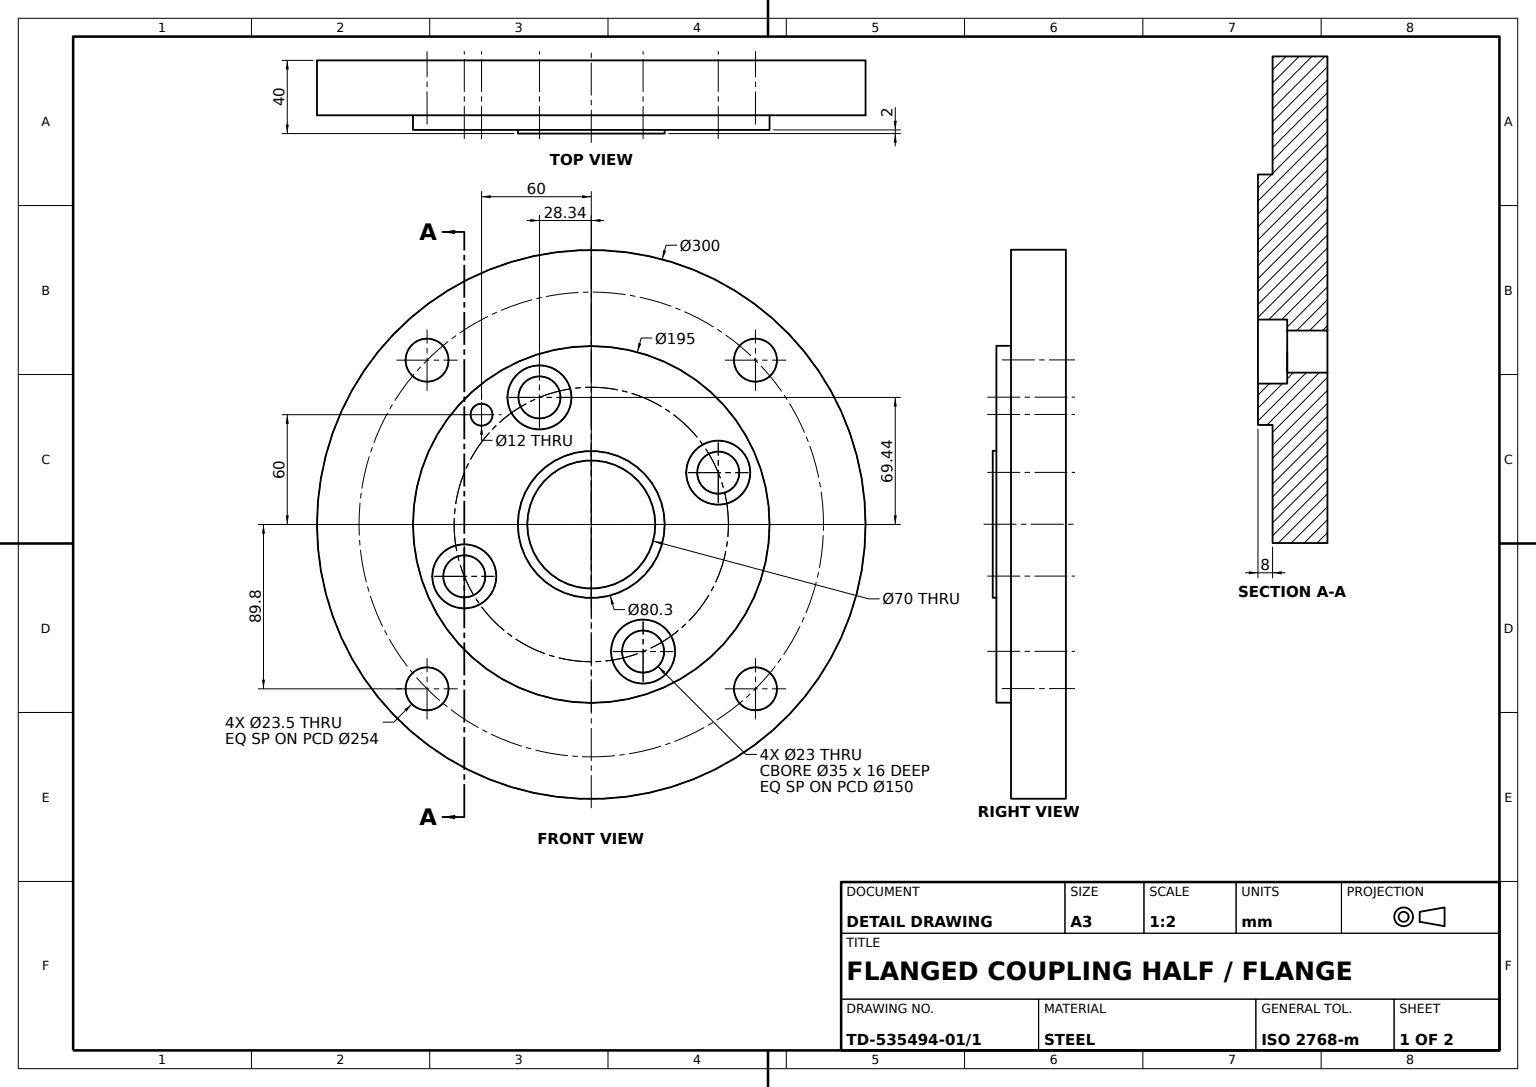
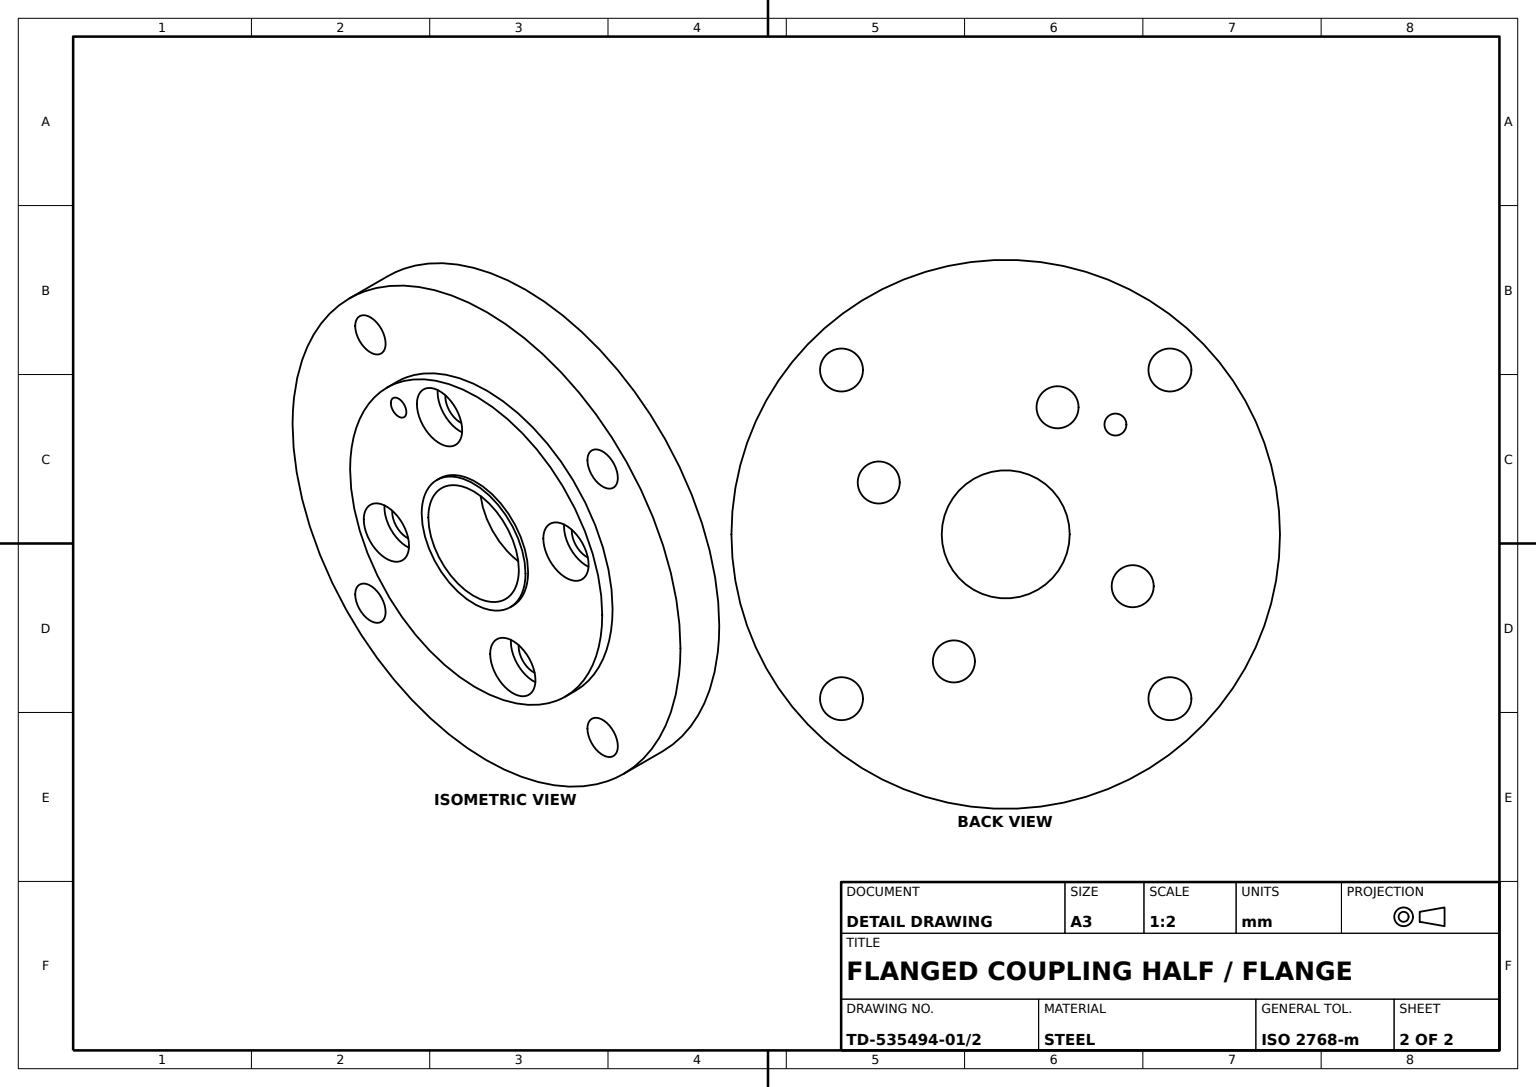
from build123d import *

# Parameters (mm, degrees)
FLANGE_DISC_PROFILE_R          = 150
FLANGE_DISC_300_DEPTH          = 30
RAISED_FACE_PROFILE_R          = 97.5
RAISED_FACE_195_DEPTH          = 8
HUB_SPIGOT_PROFILE_R           = 40.15
HUB_SPIGOT_80_3_DEPTH          = 2
THROUGH_HOLES_PROFILE_R        = 6
THROUGH_HOLES_PROFILE_R_2      = 11.75
THROUGH_HOLES_PCD254_DEPTH     = 40
COUNTERBORE_PROFILE_R          = 17.5
COUNTERBORES_4X_35_DEPTH       = 16
COUNTERBORED_HOLES_PROFILE_R   = 11.5
COUNTERBORED_HOLES_4X_23_DEPTH = 30
CENTRAL_BORE_PROFILE_R         = 35
CENTRAL_BORE_70_DEPTH          = 50


with BuildPart() as part:
    # Flange Disc Profile → Flange Disc Ø300 (new body)
    with BuildSketch(Plane.XY):
        Circle(FLANGE_DISC_PROFILE_R)
    extrude(amount=FLANGE_DISC_300_DEPTH)

    # Raised Face Profile → Raised Face Ø195 (add)
    with BuildSketch(Plane.XY.offset(30)):
        Circle(RAISED_FACE_PROFILE_R)
    extrude(amount=RAISED_FACE_195_DEPTH)

    # Hub Spigot Profile → Hub Spigot Ø80.3 (add)
    with BuildSketch(Plane.XY.offset(38)):
        Circle(HUB_SPIGOT_PROFILE_R)
    extrude(amount=HUB_SPIGOT_80_3_DEPTH)

    # Through Holes Profile → Through Holes PCD254 (cut)
    with BuildSketch(Plane.XY.offset(40)):
        with Locations((-60, 60)):
            Circle(THROUGH_HOLES_PROFILE_R)
        with Locations((89.802561211, 89.802561211)):
            Circle(THROUGH_HOLES_PROFILE_R_2)
        with Locations((89.802561211, -89.802561211)):
            Circle(THROUGH_HOLES_PROFILE_R_2)
        with Locations((-89.802561211, -89.802561211)):
            Circle(THROUGH_HOLES_PROFILE_R_2)
        with Locations((-89.802561211, 89.802561211)):
            Circle(THROUGH_HOLES_PROFILE_R_2)
    extrude(amount=-THROUGH_HOLES_PCD254_DEPTH, mode=Mode.SUBTRACT)

    # Counterbore Profile → Counterbores 4xØ35 (cut)
    with BuildSketch(Plane.XY.offset(38)):
        with Locations((-28.338059011, 69.440293861)):
            Circle(COUNTERBORE_PROFILE_R)
        with Locations((69.440293861, 28.338059011)):
            Circle(COUNTERBORE_PROFILE_R)
        with Locations((28.338059011, -69.440293861)):
            Circle(COUNTERBORE_PROFILE_R)
        with Locations((-69.440293861, -28.338059011)):
            Circle(COUNTERBORE_PROFILE_R)
    extrude(amount=-COUNTERBORES_4X_35_DEPTH, mode=Mode.SUBTRACT)

    # Counterbored Holes Profile → Counterbored Holes 4xØ23 (cut)
    with BuildSketch(Plane.XY.offset(22)):
        with Locations((-28.338059011, 69.440293861)):
            Circle(COUNTERBORED_HOLES_PROFILE_R)
        with Locations((69.440293861, 28.338059011)):
            Circle(COUNTERBORED_HOLES_PROFILE_R)
        with Locations((28.338059011, -69.440293861)):
            Circle(COUNTERBORED_HOLES_PROFILE_R)
        with Locations((-69.440293861, -28.338059011)):
            Circle(COUNTERBORED_HOLES_PROFILE_R)
    extrude(amount=-COUNTERBORED_HOLES_4X_23_DEPTH, mode=Mode.SUBTRACT)

    # Central Bore Profile → Central Bore Ø70 (cut)
    with BuildSketch(Plane.XY.offset(40)):
        Circle(CENTRAL_BORE_PROFILE_R)
    extrude(amount=-CENTRAL_BORE_70_DEPTH, mode=Mode.SUBTRACT)


solid = part.part
